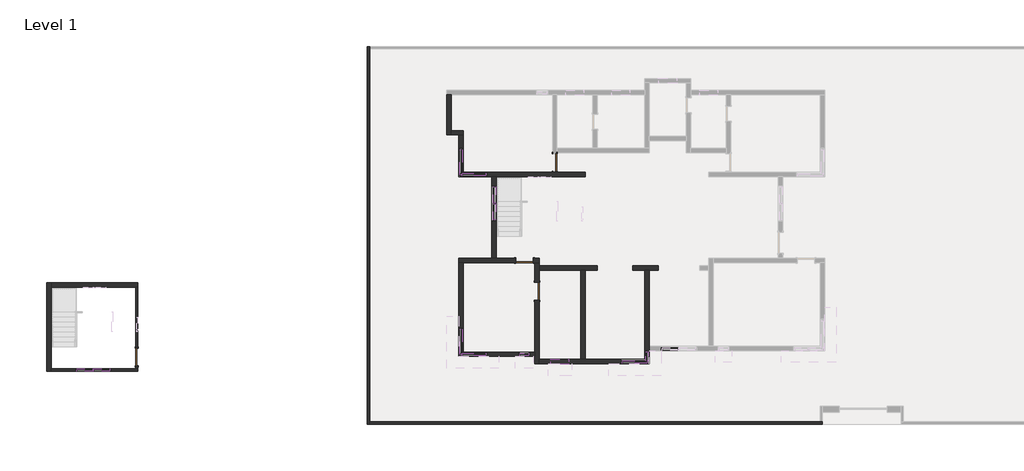
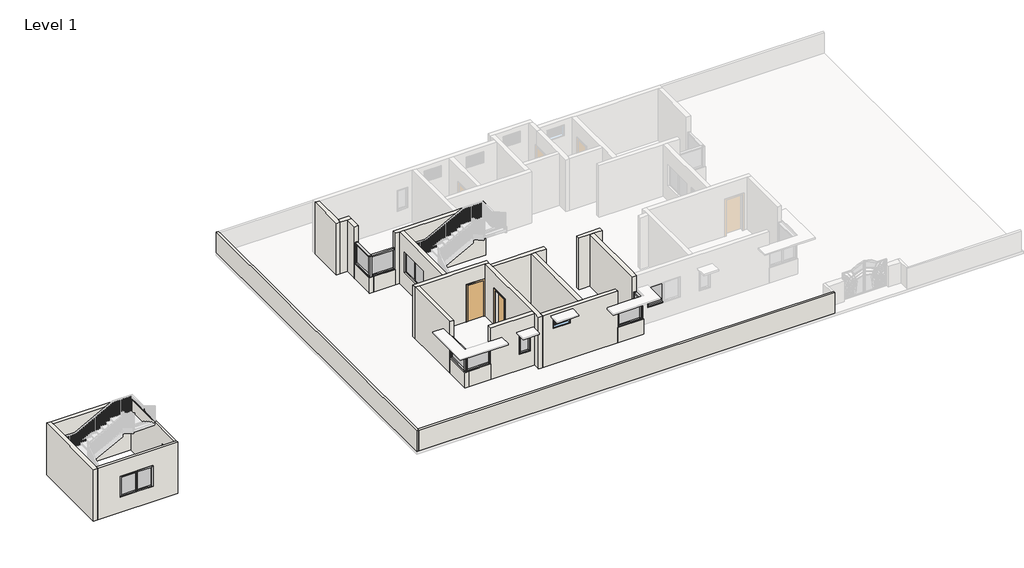
# One storey, part 1 of 9: 44 members, 26 walls, 12 plates, 4 doors, 1 window.
"""IFC4 building model written with IfcOpenShell, lengths in millimetres."""

from ifc_helpers import new_model, si_unit, frame, origin, origin_with_axes, place, context, project, spatial, polyline, outline, extrude, faceted_brep, transform, mapped, element, save
from components import single_flush_door_3_0ca8825f, single_flush_door_3_a90ba1ad, single_flush_door_3_305aa2a5, member_75074519, member_05917e3b, member_5783932f, member_d3e05364, member_2b49869a, member_9dc65bc2, member_c17f1be2, member_8d24a278, member_86d06fe4, system_panel_glazed_ffa60984, system_panel_glazed_87944ff9, system_panel_glazed_c8a97ecb, system_panel_glazed_fba3dfff, system_panel_glazed_90898af3, system_panel_glazed_d6173012, system_panel_glazed_7cebc396, system_panel_glazed_1bcf12e0, window_a18e4be4

model = new_model("IFC4")

# Units and contexts
model_context = context("Model", 3, world=origin())
ifc_project = project(units=[si_unit("LENGTHUNIT", "METRE", prefix="MILLI")], contexts=[model_context])

# Site, building, storey
site = spatial("IfcSite", under=ifc_project)
building = spatial("IfcBuilding", under=site)
storey = spatial("IfcBuildingStorey", under=building, Name="Level 1", Elevation=0.0)

# Doors
placement = place(None, origin())
single_flush_door_3_shape = single_flush_door_3_0ca8825f(model_context)
element("IfcDoor", 1, ObjectType="Single-Flush : door 3'", at=placement, inside=storey, context=model_context, shape_type="MappedRepresentation", body=[
    mapped(single_flush_door_3_shape, transform((-37991.8146233, 16182.7641869, 0.0), x_axis=(0.0, -1.0, 0.0), y_axis=(1.0, 0.0, 0.0), z_axis=(0.0, 0.0, 1.0))),
])
single_flush_door_3_2_shape = single_flush_door_3_a90ba1ad(model_context)
element("IfcDoor", 2, ObjectType="Single-Flush : door 3'", at=placement, inside=storey, context=model_context, shape_type="MappedRepresentation", body=[
    mapped(single_flush_door_3_2_shape, transform((-39541.2146233, 11158.0624892, 0.0), x_axis=(1.0, 0.0, 0.0), y_axis=(0.0, 1.0, 0.0), z_axis=(0.0, 0.0, 1.0))),
])
element("IfcDoor", 3, ObjectType="Single-Flush : door 3'", at=placement, inside=storey, context=model_context, shape_type="MappedRepresentation", body=[
    mapped(single_flush_door_3_2_shape, transform((-38906.2146233, 9583.2624892, 0.0), x_axis=(0.0, 1.0, 0.0), y_axis=(-1.0, 0.0, 0.0), z_axis=(0.0, 0.0, 1.0))),
])
single_flush_door_3_3_shape = single_flush_door_3_305aa2a5(model_context)
element("IfcDoor", 4, ObjectType="Single-Flush : door 3'", at=placement, inside=storey, context=model_context, shape_type="MappedRepresentation", body=[
    mapped(single_flush_door_3_3_shape, transform((-59414.6056789, 6214.5699577, 0.0), x_axis=(0.0, -1.0, 0.0), y_axis=(1.0, 0.0, 0.0), z_axis=(0.0, 0.0, 1.0))),
])

# Members
member_shape = member_75074519(model_context)
element("IfcMember", 5, ObjectType="Rectangular Mullion : 2.5\" x 5\" rectangular", at=placement, inside=storey, context=model_context, shape_type="MappedRepresentation", body=[
    mapped(member_shape, transform((-42808.6969478, 6281.2624892, 914.4), x_axis=(0.0, -1.0, 0.0), y_axis=(-1.0, 0.0, 0.0), z_axis=(0.0, 0.0, -1.0))),
])
element("IfcMember", 6, ObjectType="Rectangular Mullion : 2.5\" x 5\" rectangular", at=placement, inside=storey, context=model_context, shape_type="MappedRepresentation", body=[
    mapped(member_shape, transform((-41458.9146233, 6344.7624892, 914.4), x_axis=(1.0, 0.0, 0.0), y_axis=(0.0, -1.0, 0.0), z_axis=(0.0, 0.0, -1.0))),
])
element("IfcMember", 7, ObjectType="Rectangular Mullion : 2.5\" x 5\" rectangular", at=placement, inside=storey, context=model_context, shape_type="MappedRepresentation", body=[
    mapped(member_shape, transform((-42808.6027511, 15496.1692799, 914.4), x_axis=(0.0, -1.0, 0.0), y_axis=(-1.0, 0.0, 0.0), z_axis=(0.0, 0.0, -1.0))),
])
element("IfcMember", 8, ObjectType="Rectangular Mullion : 2.5\" x 5\" rectangular", at=placement, inside=storey, context=model_context, shape_type="MappedRepresentation", body=[
    mapped(member_shape, transform((-41458.9146233, 15559.6692799, 914.4), x_axis=(1.0, 0.0, 0.0), y_axis=(0.0, -1.0, 0.0), z_axis=(0.0, 0.0, -1.0))),
])
element("IfcMember", 9, ObjectType="Rectangular Mullion : 2.5\" x 5\" rectangular", at=placement, inside=storey, context=model_context, shape_type="MappedRepresentation", body=[
    mapped(member_shape, transform((-33191.2146233, 5950.984083, 914.4), x_axis=(1.0, 0.0, 0.0), y_axis=(0.0, -1.0, 0.0), z_axis=(0.0, 0.0, -1.0))),
])
element("IfcMember", 10, ObjectType="Rectangular Mullion : 2.5\" x 5\" rectangular", at=placement, inside=storey, context=model_context, shape_type="MappedRepresentation", body=[
    mapped(member_shape, transform((-33254.7146233, 6547.9624892, 914.4), x_axis=(0.0, 1.0, 0.0), y_axis=(1.0, 0.0, 0.0), z_axis=(0.0, 0.0, -1.0))),
])
element("IfcMember", 11, ObjectType="Rectangular Mullion : 2.5\" x 5\" rectangular", at=placement, inside=storey, context=model_context, shape_type="MappedRepresentation", body=[
    mapped(member_shape, transform((-41090.5055559, 15005.5684528, 914.4), x_axis=(0.0, 1.0, 0.0), y_axis=(1.0, 0.0, 0.0), z_axis=(0.0, 0.0, -1.0))),
])
element("IfcMember", 12, ObjectType="Rectangular Mullion : 2.5\" x 5\" rectangular", at=placement, inside=storey, context=model_context, shape_type="MappedRepresentation", body=[
    mapped(member_shape, transform((-60729.0556789, 5540.3224813, 914.4), x_axis=(1.0, 0.0, 0.0), y_axis=(0.0, -1.0, 0.0), z_axis=(0.0, 0.0, -1.0))),
])
element("IfcMember", 13, ObjectType="Rectangular Mullion : 2.5\" x 5\" rectangular", at=placement, inside=storey, context=model_context, shape_type="MappedRepresentation", body=[
    mapped(member_shape, transform((-39249.1146233, 6332.0624892, 914.4), x_axis=(1.0, 0.0, 0.0), y_axis=(0.0, -1.0, 0.0), z_axis=(0.0, 0.0, -1.0))),
])
element("IfcMember", 14, ObjectType="Rectangular Mullion : 2.5\" x 5\" rectangular", at=placement, inside=storey, context=model_context, shape_type="MappedRepresentation", body=[
    mapped(member_shape, transform((-42808.6969478, 7690.9624892, 2133.6), x_axis=(0.0, 1.0, 0.0), y_axis=(-1.0, 0.0, 0.0), z_axis=(0.0, 0.0, 1.0))),
])
element("IfcMember", 15, ObjectType="Rectangular Mullion : 2.5\" x 5\" rectangular", at=placement, inside=storey, context=model_context, shape_type="MappedRepresentation", body=[
    mapped(member_shape, transform((-42808.6969478, 6344.7624892, 2133.6), x_axis=(-1.0, 0.0, 0.0), y_axis=(0.0, -1.0, 0.0), z_axis=(0.0, 0.0, 1.0))),
])
element("IfcMember", 16, ObjectType="Rectangular Mullion : 2.5\" x 5\" rectangular", at=placement, inside=storey, context=model_context, shape_type="MappedRepresentation", body=[
    mapped(member_shape, transform((-42808.6027511, 16911.1624892, 2133.6), x_axis=(0.0, 1.0, 0.0), y_axis=(-1.0, 0.0, 0.0), z_axis=(0.0, 0.0, 1.0))),
])
element("IfcMember", 17, ObjectType="Rectangular Mullion : 2.5\" x 5\" rectangular", at=placement, inside=storey, context=model_context, shape_type="MappedRepresentation", body=[
    mapped(member_shape, transform((-42808.6027511, 15559.6692799, 2133.6), x_axis=(-1.0, 0.0, 0.0), y_axis=(0.0, -1.0, 0.0), z_axis=(0.0, 0.0, 1.0))),
])
element("IfcMember", 18, ObjectType="Rectangular Mullion : 2.5\" x 5\" rectangular", at=placement, inside=storey, context=model_context, shape_type="MappedRepresentation", body=[
    mapped(member_shape, transform((-34600.9146233, 5950.984083, 2133.6), x_axis=(-1.0, 0.0, 0.0), y_axis=(0.0, -1.0, 0.0), z_axis=(0.0, 0.0, 1.0))),
])
element("IfcMember", 19, ObjectType="Rectangular Mullion : 2.5\" x 5\" rectangular", at=placement, inside=storey, context=model_context, shape_type="MappedRepresentation", body=[
    mapped(member_shape, transform((-33254.7146233, 5950.984083, 2133.6), x_axis=(0.0, -1.0, 0.0), y_axis=(1.0, 0.0, 0.0), z_axis=(0.0, 0.0, 1.0))),
])
element("IfcMember", 20, ObjectType="Rectangular Mullion : 2.5\" x 5\" rectangular", at=placement, inside=storey, context=model_context, shape_type="MappedRepresentation", body=[
    mapped(member_shape, transform((-32543.5146233, 6636.8624892, 2133.6), x_axis=(-1.0, 0.0, 0.0), y_axis=(0.0, -1.0, 0.0), z_axis=(0.0, 0.0, 1.0))),
])
element("IfcMember", 21, ObjectType="Rectangular Mullion : 2.5\" x 5\" rectangular", at=placement, inside=storey, context=model_context, shape_type="MappedRepresentation", body=[
    mapped(member_shape, transform((-41090.5055559, 13177.3624892, 2133.6), x_axis=(0.0, -1.0, 0.0), y_axis=(1.0, 0.0, 0.0), z_axis=(0.0, 0.0, 1.0))),
])
element("IfcMember", 22, ObjectType="Rectangular Mullion : 2.5\" x 5\" rectangular", at=placement, inside=storey, context=model_context, shape_type="MappedRepresentation", body=[
    mapped(member_shape, transform((-62557.8556789, 5540.3224813, 2133.6), x_axis=(-1.0, 0.0, 0.0), y_axis=(0.0, -1.0, 0.0), z_axis=(0.0, 0.0, 1.0))),
])
element("IfcMember", 23, ObjectType="Rectangular Mullion : 2.5\" x 5\" rectangular", at=placement, inside=storey, context=model_context, shape_type="MappedRepresentation", body=[
    mapped(member_shape, transform((-39858.7146233, 6332.0624892, 2133.6), x_axis=(-1.0, 0.0, 0.0), y_axis=(0.0, -1.0, 0.0), z_axis=(0.0, 0.0, 1.0))),
])
member_2_shape = member_05917e3b(model_context)
element("IfcMember", 24, ObjectType="Rectangular Mullion : 2.5\" x 5\" rectangular", at=placement, inside=storey, context=model_context, shape_type="MappedRepresentation", body=[
    mapped(member_2_shape, transform((-41522.4146233, 6344.7624892, 2133.6), x_axis=(0.0, 0.0, 1.0), y_axis=(0.0, -1.0, 0.0), z_axis=(1.0, 0.0, 0.0))),
])
element("IfcMember", 25, ObjectType="Rectangular Mullion : 2.5\" x 5\" rectangular", at=placement, inside=storey, context=model_context, shape_type="MappedRepresentation", body=[
    mapped(member_2_shape, transform((-41522.4146233, 15559.6692799, 2133.6), x_axis=(0.0, 0.0, 1.0), y_axis=(0.0, -1.0, 0.0), z_axis=(1.0, 0.0, 0.0))),
])
element("IfcMember", 26, ObjectType="Rectangular Mullion : 2.5\" x 5\" rectangular", at=placement, inside=storey, context=model_context, shape_type="MappedRepresentation", body=[
    mapped(member_2_shape, transform((-42745.1969478, 6344.7624892, 914.4), x_axis=(0.0, 0.0, -1.0), y_axis=(0.0, -1.0, 0.0), z_axis=(-1.0, 0.0, 0.0))),
])
element("IfcMember", 27, ObjectType="Rectangular Mullion : 2.5\" x 5\" rectangular", at=placement, inside=storey, context=model_context, shape_type="MappedRepresentation", body=[
    mapped(member_2_shape, transform((-42745.1027511, 15559.6692799, 914.4), x_axis=(0.0, 0.0, -1.0), y_axis=(0.0, -1.0, 0.0), z_axis=(-1.0, 0.0, 0.0))),
])
member_3_shape = member_5783932f(model_context)
element("IfcMember", 28, ObjectType="Rectangular Mullion : 2.5\" x 5\" rectangular", at=placement, inside=storey, context=model_context, shape_type="MappedRepresentation", body=[
    mapped(member_3_shape, transform((-42808.6969478, 6344.7624892, 2133.6), x_axis=(0.0, 0.0, 1.0), y_axis=(-1.0, 0.0, 0.0), z_axis=(0.0, -1.0, 0.0))),
])
element("IfcMember", 29, ObjectType="Rectangular Mullion : 2.5\" x 5\" rectangular", at=placement, inside=storey, context=model_context, shape_type="MappedRepresentation", body=[
    mapped(member_3_shape, transform((-33254.7146233, 5950.984083, 2133.6), x_axis=(0.0, 0.0, 1.0), y_axis=(0.0, -1.0, 0.0), z_axis=(1.0, 0.0, 0.0))),
])
element("IfcMember", 30, ObjectType="Rectangular Mullion : 2.5\" x 5\" rectangular", at=placement, inside=storey, context=model_context, shape_type="MappedRepresentation", body=[
    mapped(member_3_shape, transform((-42808.6969478, 7627.4624892, 914.4), x_axis=(0.0, 0.0, -1.0), y_axis=(-1.0, 0.0, 0.0), z_axis=(0.0, 1.0, 0.0))),
])
element("IfcMember", 31, ObjectType="Rectangular Mullion : 2.5\" x 5\" rectangular", at=placement, inside=storey, context=model_context, shape_type="MappedRepresentation", body=[
    mapped(member_3_shape, transform((-34537.4146233, 5950.984083, 914.4), x_axis=(0.0, 0.0, -1.0), y_axis=(0.0, -1.0, 0.0), z_axis=(-1.0, 0.0, 0.0))),
])
member_4_shape = member_d3e05364(model_context)
element("IfcMember", 32, ObjectType="Rectangular Mullion : 2.5\" x 5\" rectangular", at=placement, inside=storey, context=model_context, shape_type="MappedRepresentation", body=[
    mapped(member_4_shape, transform((-42808.6027511, 15559.6692799, 2133.6), x_axis=(0.0, 0.0, 1.0), y_axis=(-1.0, 0.0, 0.0), z_axis=(0.0, -1.0, 0.0))),
])
element("IfcMember", 33, ObjectType="Rectangular Mullion : 2.5\" x 5\" rectangular", at=placement, inside=storey, context=model_context, shape_type="MappedRepresentation", body=[
    mapped(member_4_shape, transform((-42808.6027511, 16847.6624892, 914.4), x_axis=(0.0, 0.0, -1.0), y_axis=(-1.0, 0.0, 0.0), z_axis=(0.0, 1.0, 0.0))),
])
member_5_shape = member_2b49869a(model_context)
element("IfcMember", 34, ObjectType="Rectangular Mullion : 2.5\" x 5\" rectangular", at=placement, inside=storey, context=model_context, shape_type="MappedRepresentation", body=[
    mapped(member_5_shape, transform((-41090.5055559, 14091.465471, 914.4), x_axis=(0.0, 1.0, 0.0), y_axis=(1.0, 0.0, 0.0), z_axis=(0.0, 0.0, -1.0))),
])
element("IfcMember", 35, ObjectType="Rectangular Mullion : 2.5\" x 5\" rectangular", at=placement, inside=storey, context=model_context, shape_type="MappedRepresentation", body=[
    mapped(member_5_shape, transform((-61643.4556789, 5540.3224813, 914.4), x_axis=(1.0, 0.0, 0.0), y_axis=(0.0, -1.0, 0.0), z_axis=(0.0, 0.0, -1.0))),
])
member_6_shape = member_9dc65bc2(model_context)
element("IfcMember", 36, ObjectType="Rectangular Mullion : 2.5\" x 5\" rectangular", at=placement, inside=storey, context=model_context, shape_type="MappedRepresentation", body=[
    mapped(member_6_shape, transform((-33254.7146233, 6484.4624892, 2133.6), x_axis=(0.0, 0.0, 1.0), y_axis=(1.0, 0.0, 0.0), z_axis=(0.0, 1.0, 0.0))),
])
element("IfcMember", 37, ObjectType="Rectangular Mullion : 2.5\" x 5\" rectangular", at=placement, inside=storey, context=model_context, shape_type="MappedRepresentation", body=[
    mapped(member_6_shape, transform((-33254.7146233, 6014.484083, 914.4), x_axis=(0.0, 0.0, -1.0), y_axis=(1.0, 0.0, 0.0), z_axis=(0.0, -1.0, 0.0))),
])
member_7_shape = member_c17f1be2(model_context)
element("IfcMember", 38, ObjectType="Rectangular Mullion : 2.5\" x 5\" rectangular", at=placement, inside=storey, context=model_context, shape_type="MappedRepresentation", body=[
    mapped(member_7_shape, transform((-60792.5556789, 5540.3224813, 2133.6), x_axis=(0.0, 0.0, 1.0), y_axis=(0.0, -1.0, 0.0), z_axis=(1.0, 0.0, 0.0))),
])
element("IfcMember", 39, ObjectType="Rectangular Mullion : 2.5\" x 5\" rectangular", at=placement, inside=storey, context=model_context, shape_type="MappedRepresentation", body=[
    mapped(member_7_shape, transform((-61675.2056789, 5540.3224813, 2133.6), x_axis=(0.0, 0.0, 1.0), y_axis=(0.0, -1.0, 0.0), z_axis=(1.0, 0.0, 0.0))),
])
element("IfcMember", 40, ObjectType="Rectangular Mullion : 2.5\" x 5\" rectangular", at=placement, inside=storey, context=model_context, shape_type="MappedRepresentation", body=[
    mapped(member_7_shape, transform((-32480.0146233, 6636.8624892, 914.4), x_axis=(0.0, 0.0, -1.0), y_axis=(0.0, -1.0, 0.0), z_axis=(-1.0, 0.0, 0.0))),
])
element("IfcMember", 41, ObjectType="Rectangular Mullion : 2.5\" x 5\" rectangular", at=placement, inside=storey, context=model_context, shape_type="MappedRepresentation", body=[
    mapped(member_7_shape, transform((-62494.3556789, 5540.3224813, 914.4), x_axis=(0.0, 0.0, -1.0), y_axis=(0.0, -1.0, 0.0), z_axis=(-1.0, 0.0, 0.0))),
])
element("IfcMember", 42, ObjectType="Rectangular Mullion : 2.5\" x 5\" rectangular", at=placement, inside=storey, context=model_context, shape_type="MappedRepresentation", body=[
    mapped(member_7_shape, transform((-61611.7056789, 5540.3224813, 914.4), x_axis=(0.0, 0.0, -1.0), y_axis=(0.0, -1.0, 0.0), z_axis=(-1.0, 0.0, 0.0))),
])
member_8_shape = member_8d24a278(model_context)
element("IfcMember", 43, ObjectType="Rectangular Mullion : 2.5\" x 5\" rectangular", at=placement, inside=storey, context=model_context, shape_type="MappedRepresentation", body=[
    mapped(member_8_shape, transform((-41090.5055559, 14942.0684528, 2133.6), x_axis=(0.0, 0.0, 1.0), y_axis=(1.0, 0.0, 0.0), z_axis=(0.0, 1.0, 0.0))),
])
element("IfcMember", 44, ObjectType="Rectangular Mullion : 2.5\" x 5\" rectangular", at=placement, inside=storey, context=model_context, shape_type="MappedRepresentation", body=[
    mapped(member_8_shape, transform((-41090.5055559, 14059.715471, 2133.6), x_axis=(0.0, 0.0, 1.0), y_axis=(1.0, 0.0, 0.0), z_axis=(0.0, 1.0, 0.0))),
])
element("IfcMember", 45, ObjectType="Rectangular Mullion : 2.5\" x 5\" rectangular", at=placement, inside=storey, context=model_context, shape_type="MappedRepresentation", body=[
    mapped(member_8_shape, transform((-41090.5055559, 13240.8624892, 914.4), x_axis=(0.0, 0.0, -1.0), y_axis=(1.0, 0.0, 0.0), z_axis=(0.0, -1.0, 0.0))),
])
element("IfcMember", 46, ObjectType="Rectangular Mullion : 2.5\" x 5\" rectangular", at=placement, inside=storey, context=model_context, shape_type="MappedRepresentation", body=[
    mapped(member_8_shape, transform((-41090.5055559, 14123.215471, 914.4), x_axis=(0.0, 0.0, -1.0), y_axis=(1.0, 0.0, 0.0), z_axis=(0.0, -1.0, 0.0))),
])
member_9_shape = member_86d06fe4(model_context)
element("IfcMember", 47, ObjectType="Rectangular Mullion : 2.5\" x 5\" rectangular", at=placement, inside=storey, context=model_context, shape_type="MappedRepresentation", body=[
    mapped(member_9_shape, transform((-39312.6146233, 6332.0624892, 2133.6), x_axis=(0.0, 0.0, 1.0), y_axis=(0.0, -1.0, 0.0), z_axis=(1.0, 0.0, 0.0))),
])
element("IfcMember", 48, ObjectType="Rectangular Mullion : 2.5\" x 5\" rectangular", at=placement, inside=storey, context=model_context, shape_type="MappedRepresentation", body=[
    mapped(member_9_shape, transform((-39795.2146233, 6332.0624892, 914.4), x_axis=(0.0, 0.0, -1.0), y_axis=(0.0, -1.0, 0.0), z_axis=(-1.0, 0.0, 0.0))),
])

# Plates
system_panel_glazed_shape = system_panel_glazed_ffa60984(model_context)
element("IfcPlate", 49, ObjectType="System Panel : Glazed", at=placement, inside=storey, context=model_context, shape_type="MappedRepresentation", body=[
    mapped(system_panel_glazed_shape, transform((-42133.8057856, 6344.7624892, 977.9), x_axis=(1.0, 0.0, 0.0), y_axis=(0.0, 1.0, 0.0), z_axis=(0.0, 0.0, 1.0))),
])
system_panel_glazed_2_shape = system_panel_glazed_87944ff9(model_context)
element("IfcPlate", 50, ObjectType="System Panel : Glazed", at=placement, inside=storey, context=model_context, shape_type="MappedRepresentation", body=[
    mapped(system_panel_glazed_2_shape, transform((-42808.6969478, 6986.1124892, 977.9), x_axis=(0.0, -1.0, 0.0), y_axis=(1.0, 0.0, 0.0), z_axis=(0.0, 0.0, 1.0))),
])
element("IfcPlate", 51, ObjectType="System Panel : Glazed", at=placement, inside=storey, context=model_context, shape_type="MappedRepresentation", body=[
    mapped(system_panel_glazed_2_shape, transform((-33896.0646233, 5950.984083, 977.9), x_axis=(1.0, 0.0, 0.0), y_axis=(0.0, 1.0, 0.0), z_axis=(0.0, 0.0, 1.0))),
])
system_panel_glazed_3_shape = system_panel_glazed_c8a97ecb(model_context)
element("IfcPlate", 52, ObjectType="System Panel : Glazed", at=placement, inside=storey, context=model_context, shape_type="MappedRepresentation", body=[
    mapped(system_panel_glazed_3_shape, transform((-42133.7586872, 15559.6692799, 977.9), x_axis=(1.0, 0.0, 0.0), y_axis=(0.0, 1.0, 0.0), z_axis=(0.0, 0.0, 1.0))),
])
system_panel_glazed_4_shape = system_panel_glazed_fba3dfff(model_context)
element("IfcPlate", 53, ObjectType="System Panel : Glazed", at=placement, inside=storey, context=model_context, shape_type="MappedRepresentation", body=[
    mapped(system_panel_glazed_4_shape, transform((-42808.6027511, 16203.6658846, 977.9), x_axis=(0.0, -1.0, 0.0), y_axis=(1.0, 0.0, 0.0), z_axis=(0.0, 0.0, 1.0))),
])
system_panel_glazed_5_shape = system_panel_glazed_90898af3(model_context)
element("IfcPlate", 54, ObjectType="System Panel : Glazed", at=placement, inside=storey, context=model_context, shape_type="MappedRepresentation", body=[
    mapped(system_panel_glazed_5_shape, transform((-33254.7146233, 6249.4732861, 977.9), x_axis=(0.0, 1.0, 0.0), y_axis=(-1.0, 0.0, 0.0), z_axis=(0.0, 0.0, 1.0))),
])
system_panel_glazed_6_shape = system_panel_glazed_d6173012(model_context)
element("IfcPlate", 55, ObjectType="System Panel : Glazed", at=placement, inside=storey, context=model_context, shape_type="MappedRepresentation", body=[
    mapped(system_panel_glazed_6_shape, transform((-32070.4396233, 6636.8624892, 977.9), x_axis=(1.0, 0.0, 0.0), y_axis=(0.0, 1.0, 0.0), z_axis=(0.0, 0.0, 1.0))),
])
element("IfcPlate", 56, ObjectType="System Panel : Glazed", at=placement, inside=storey, context=model_context, shape_type="MappedRepresentation", body=[
    mapped(system_panel_glazed_6_shape, transform((-62084.7806789, 5540.3224813, 977.9), x_axis=(1.0, 0.0, 0.0), y_axis=(0.0, 1.0, 0.0), z_axis=(0.0, 0.0, 1.0))),
])
element("IfcPlate", 57, ObjectType="System Panel : Glazed", at=placement, inside=storey, context=model_context, shape_type="MappedRepresentation", body=[
    mapped(system_panel_glazed_6_shape, transform((-61202.1306789, 5540.3224813, 977.9), x_axis=(1.0, 0.0, 0.0), y_axis=(0.0, 1.0, 0.0), z_axis=(0.0, 0.0, 1.0))),
])
system_panel_glazed_7_shape = system_panel_glazed_7cebc396(model_context)
element("IfcPlate", 58, ObjectType="System Panel : Glazed", at=placement, inside=storey, context=model_context, shape_type="MappedRepresentation", body=[
    mapped(system_panel_glazed_7_shape, transform((-41090.5055559, 13650.2889801, 977.9), x_axis=(0.0, 1.0, 0.0), y_axis=(-1.0, 0.0, 0.0), z_axis=(0.0, 0.0, 1.0))),
])
element("IfcPlate", 59, ObjectType="System Panel : Glazed", at=placement, inside=storey, context=model_context, shape_type="MappedRepresentation", body=[
    mapped(system_panel_glazed_7_shape, transform((-41090.5055559, 14532.6419619, 977.9), x_axis=(0.0, 1.0, 0.0), y_axis=(-1.0, 0.0, 0.0), z_axis=(0.0, 0.0, 1.0))),
])
system_panel_glazed_8_shape = system_panel_glazed_1bcf12e0(model_context)
element("IfcPlate", 60, ObjectType="System Panel : Glazed", at=placement, inside=storey, context=model_context, shape_type="MappedRepresentation", body=[
    mapped(system_panel_glazed_8_shape, transform((-39553.9146233, 6332.0624892, 977.9), x_axis=(1.0, 0.0, 0.0), y_axis=(0.0, 1.0, 0.0), z_axis=(0.0, 0.0, 1.0))),
])

# Walls
element("IfcWall", 61, at=placement, inside=storey, context=model_context, shape_type="Brep", body=[
    faceted_brep([(-47478.7146233, 2776.0624892, 0.0), (-47478.7146233, 2890.3624892, 0.0), (-47478.7146233, 22016.5624892, 0.0), (-47478.7146233, 22130.8624892, 0.0), (-47478.7146233, 22130.8624892, 1219.2), (-47478.7146233, 22016.5624892, 1219.2), (-47478.7146233, 2890.3624892, 1219.2), (-47478.7146233, 2776.0624892, 1219.2), (-47593.0146233, 2776.0624892, 0.0), (-47593.0146233, 2776.0624892, 1219.2), (-47593.0146233, 22130.8624892, 1219.2), (-47593.0146233, 22130.8624892, 0.0)], [[[0, 1, 2, 3, 4, 5, 6, 7]], [[8, 9, 10, 11]], [[3, 2, 1, 0, 8, 11]], [[7, 6, 5, 4, 10, 9]], [[4, 3, 11, 10]], [[0, 7, 9, 8]]]),
])
element("IfcWall", 62, at=placement, inside=storey, context=model_context, shape_type="Brep", body=[
    faceted_brep([(-47478.7146233, 2776.0624892, 0.0), (-24275.8146233, 2776.0624892, 0.0), (-24275.8146233, 2776.0624892, 1219.2), (-47478.7146233, 2776.0624892, 1219.2), (-47478.7146233, 2890.3624892, 0.0), (-47478.7146233, 2890.3624892, 1219.2), (-24390.1146233, 2890.3624892, 1219.2), (-24275.8146233, 2890.3624892, 1219.2), (-24275.8146233, 2890.3624892, 0.0), (-24390.1146233, 2890.3624892, 0.0)], [[[0, 1, 2, 3]], [[4, 5, 6, 7, 8, 9]], [[1, 0, 4, 9, 8]], [[3, 2, 7, 6, 5]], [[0, 3, 5, 4]], [[2, 1, 8, 7]]]),
])
element("IfcWall", 63, ObjectType="Generic - 5\"", at=placement, inside=storey, context=model_context, shape_type="Brep", body=[
    faceted_brep([(-63814.6636189, 5497.0199577, 0.0), (-59357.4556789, 5497.0199577, 0.0), (-59357.4556789, 5497.0199577, 3048.0), (-63814.6636189, 5497.0199577, 3048.0), (-62557.8556789, 5497.0199577, 914.4), (-62557.8556789, 5497.0199577, 2133.6), (-60729.0556789, 5497.0199577, 2133.6), (-60729.0556789, 5497.0199577, 914.4), (-59357.4556789, 5611.3199577, 0.0), (-59471.7556789, 5611.3199577, 0.0), (-63814.6636189, 5611.3199577, 0.0), (-63814.6636189, 5611.3199577, 3048.0), (-59471.7556789, 5611.3199577, 3048.0), (-59357.4556789, 5611.3199577, 3048.0), (-62557.8556789, 5611.3199577, 2133.6), (-62557.8556789, 5611.3199577, 914.4), (-60729.0556789, 5611.3199577, 914.4), (-60729.0556789, 5611.3199577, 2133.6)], [[[0, 1, 2, 3], [4, 5, 6, 7]], [[8, 9, 10, 11, 12, 13], [14, 15, 16, 17]], [[1, 0, 10, 9, 8]], [[2, 1, 8, 13]], [[0, 3, 11, 10]], [[4, 15, 14, 5]], [[5, 14, 17, 6]], [[6, 17, 16, 7]], [[15, 4, 7, 16]], [[3, 2, 13, 12, 11]]]),
])
element("IfcWall", 64, ObjectType="Generic - 5\"", at=placement, inside=storey, context=model_context, shape_type="Brep", body=[
    faceted_brep([(-59357.4556789, 5611.3199577, 0.0), (-59357.4556789, 5757.3699577, 0.0), (-59357.4556789, 5757.3699577, 2133.6), (-59357.4556789, 6671.7699577, 2133.6), (-59357.4556789, 6671.7699577, 0.0), (-59357.4556789, 9802.3199577, 0.0), (-59357.4556789, 9802.3199577, 3048.0), (-59357.4556789, 5611.3199577, 3048.0), (-59471.7556789, 5757.3699577, 2133.6), (-59471.7556789, 5757.3699577, 0.0), (-59471.7556789, 5611.3199577, 0.0), (-59471.7556789, 5611.3199577, 3048.0), (-59471.7556789, 9802.3199577, 3048.0), (-59471.7556789, 9802.3199577, 0.0), (-59471.7556789, 6671.7699577, 0.0), (-59471.7556789, 6671.7699577, 2133.6), (-59471.2636189, 5611.3199577, 3048.0), (-59471.2636189, 9802.3199577, 3048.0), (-59471.2636189, 7516.3199577, 3048.0)], [[[0, 1, 2, 3, 4, 5, 6, 7]], [[8, 9, 10, 11, 12, 13, 14, 15]], [[14, 13, 5, 4]], [[10, 9, 1, 0]], [[0, 7, 16, 11, 10]], [[6, 5, 13, 12, 17]], [[2, 1, 9, 8]], [[3, 2, 8, 15]], [[4, 3, 15, 14]], [[7, 6, 17, 18, 16]], [[17, 12, 11, 16, 18]]]),
])
element("IfcWall", 65, ObjectType="WALL 9\" 2", at=placement, inside=storey, context=model_context, shape_type="Brep", body=[
    faceted_brep([(-43516.3146233, 19654.3624892, 0.0), (-43516.3146233, 17596.9624892, 0.0), (-43516.3146233, 17596.9624892, 3048.0), (-43516.3146233, 19654.3624892, 3048.0), (-43287.7146233, 19654.3624892, 0.0), (-43287.7146233, 19654.3624892, 3048.0), (-43287.7146233, 17825.5624892, 3048.0), (-43287.7146233, 17596.9624892, 3048.0), (-43287.7146233, 17596.9624892, 0.0), (-43287.7146233, 17825.5624892, 0.0)], [[[0, 1, 2, 3]], [[4, 5, 6, 7, 8, 9]], [[1, 0, 4, 9, 8]], [[3, 2, 7, 6, 5]], [[0, 3, 5, 4]], [[2, 1, 8, 7]]]),
])
element("IfcWall", 66, ObjectType="WALL 9\" 2", at=placement, inside=storey, context=model_context, shape_type="Brep", body=[
    faceted_brep([(-43287.7146233, 17596.9624892, 0.0), (-42906.7146233, 17596.9624892, 0.0), (-42678.1146233, 17596.9624892, 0.0), (-42678.1146233, 17596.9624892, 3048.0), (-42906.7146233, 17596.9624892, 3048.0), (-43287.7146233, 17596.9624892, 3048.0), (-43287.7146233, 17825.5624892, 0.0), (-43287.7146233, 17825.5624892, 3048.0), (-42678.1146233, 17825.5624892, 3048.0), (-42678.1146233, 17825.5624892, 0.0)], [[[0, 1, 2, 3, 4, 5]], [[6, 7, 8, 9]], [[2, 1, 0, 6, 9]], [[5, 4, 3, 8, 7]], [[0, 5, 7, 6]], [[3, 2, 9, 8]]]),
])
element("IfcWall", 67, ObjectType="WALL 9\" 2", at=placement, inside=storey, context=model_context, shape_type="Brep", body=[
    faceted_brep([(-42906.7146233, 17596.9624892, 0.0), (-42906.7146233, 16911.1624892, 0.0), (-42906.7146233, 16911.1624892, 914.4), (-42906.7146233, 16911.1624892, 2133.6), (-42906.7146233, 16911.1624892, 3048.0), (-42906.7146233, 17596.9624892, 3048.0), (-42678.1146233, 17596.9624892, 0.0), (-42678.1146233, 17596.9624892, 3048.0), (-42678.1146233, 16911.1624892, 3048.0), (-42678.1146233, 16911.1624892, 2133.6), (-42678.1146233, 16911.1624892, 914.4), (-42678.1146233, 16911.1624892, 0.0)], [[[0, 1, 2, 3, 4, 5]], [[6, 7, 8, 9, 10, 11]], [[1, 0, 6, 11]], [[5, 4, 8, 7]], [[0, 5, 7, 6]], [[1, 11, 10, 9, 8, 4, 3, 2]]]),
])
element("IfcWall", 68, ObjectType="WALL 9\" 2", at=placement, inside=storey, context=model_context, shape_type="Brep", body=[
    faceted_brep([(-41458.9146233, 15454.3658846, 3048.0), (-41458.9146233, 15454.3658846, 2133.6), (-41458.9146233, 15454.3658846, 914.4), (-41458.9146233, 15454.3658846, 0.0), (-41230.3146233, 15454.3658846, 0.0), (-41001.7146233, 15454.3658846, 0.0), (-36429.7146233, 15454.3658846, 0.0), (-36429.7146233, 15454.3658846, 3048.0), (-41001.7146233, 15454.3658846, 3048.0), (-41230.3146233, 15454.3658846, 3048.0), (-41458.9146233, 15682.9658846, 0.0), (-41458.9146233, 15682.9658846, 914.4), (-41458.9146233, 15682.9658846, 2133.6), (-41458.9146233, 15682.9658846, 3048.0), (-38106.1146233, 15682.9658846, 3048.0), (-37877.5146233, 15682.9658846, 3048.0), (-36429.7146233, 15682.9658846, 3048.0), (-36429.7146233, 15682.9658846, 0.0), (-37877.5146233, 15682.9658846, 0.0), (-38106.1146233, 15682.9658846, 0.0)], [[[0, 1, 2, 3, 4, 5, 6, 7, 8, 9]], [[10, 11, 12, 13, 14, 15, 16, 17, 18, 19]], [[6, 5, 4, 3, 10, 19, 18, 17]], [[7, 6, 17, 16]], [[0, 9, 8, 7, 16, 15, 14, 13]], [[0, 13, 12, 11, 10, 3, 2, 1]]]),
])
element("IfcWall", 69, ObjectType="WALL 9\" 2", at=placement, inside=storey, context=model_context, shape_type="SweptSolid", body=[
    extrude(outline(polyline([(15454.3658846, 0.0), (11272.3624892, 0.0), (11272.3624892, 3048.0), (15454.3658846, 3048.0), (15454.3658846, 0.0)]), holes=[polyline([(13177.3624892, 2133.6), (13177.3624892, 914.4), (15005.5684528, 914.4), (15005.5684528, 2133.6), (13177.3624892, 2133.6)])]), frame((-41230.3146233, 0.0, 0.0), z_axis=(1.0, 0.0, 0.0), x_axis=(0.0, 1.0, 0.0)), (0.0, 0.0, 1.0), 228.6),
])
element("IfcWall", 70, ObjectType="WALL 9\" 2", at=placement, inside=storey, context=model_context, shape_type="Brep", body=[
    faceted_brep([(-39084.0146233, 11043.7624892, 2133.6), (-39084.0146233, 11043.7624892, 0.0), (-39020.5146233, 11043.7624892, 0.0), (-38791.9146233, 11043.7624892, 0.0), (-38791.9146233, 11043.7624892, 3048.0), (-39020.5146233, 11043.7624892, 3048.0), (-42678.1146233, 11043.7624892, 3048.0), (-42906.7146233, 11043.7624892, 3048.0), (-42906.7146233, 11043.7624892, 0.0), (-42678.1146233, 11043.7624892, 0.0), (-39998.4146233, 11043.7624892, 0.0), (-39998.4146233, 11043.7624892, 2133.6), (-38791.9146233, 11272.3624892, 0.0), (-39084.0146233, 11272.3624892, 0.0), (-39084.0146233, 11272.3624892, 2133.6), (-39998.4146233, 11272.3624892, 2133.6), (-39998.4146233, 11272.3624892, 0.0), (-41001.7146233, 11272.3624892, 0.0), (-41230.3146233, 11272.3624892, 0.0), (-42906.7146233, 11272.3624892, 0.0), (-42906.7146233, 11272.3624892, 3048.0), (-41230.3146233, 11272.3624892, 3048.0), (-41001.7146233, 11272.3624892, 3048.0), (-38791.9146233, 11272.3624892, 3048.0)], [[[0, 1, 2, 3, 4, 5, 6, 7, 8, 9, 10, 11]], [[12, 13, 14, 15, 16, 17, 18, 19, 20, 21, 22, 23]], [[10, 9, 8, 19, 18, 17, 16]], [[3, 2, 1, 13, 12]], [[7, 6, 5, 4, 23, 22, 21, 20]], [[4, 3, 12, 23]], [[8, 7, 20, 19]], [[14, 13, 1, 0]], [[15, 14, 0, 11]], [[16, 15, 11, 10]]]),
])
element("IfcWall", 71, ObjectType="WALL 9\" 2", at=placement, inside=storey, context=model_context, shape_type="Brep", body=[
    faceted_brep([(-39020.5146233, 11043.7624892, 0.0), (-39020.5146233, 10040.4624892, 0.0), (-39020.5146233, 10040.4624892, 2133.6), (-39020.5146233, 9126.0624892, 2133.6), (-39020.5146233, 9126.0624892, 0.0), (-39020.5146233, 6471.7624892, 0.0), (-39020.5146233, 6243.1624892, 0.0), (-39020.5146233, 5862.084083, 0.0), (-39020.5146233, 5862.084083, 3048.0), (-39020.5146233, 6243.1624892, 3048.0), (-39020.5146233, 6471.7624892, 3048.0), (-39020.5146233, 11043.7624892, 3048.0), (-38791.9146233, 10040.4624892, 2133.6), (-38791.9146233, 10040.4624892, 0.0), (-38791.9146233, 10662.7624892, 0.0), (-38791.9146233, 10891.3624892, 0.0), (-38791.9146233, 11043.7624892, 0.0), (-38791.9146233, 11043.7624892, 3048.0), (-38791.9146233, 10891.3624892, 3048.0), (-38791.9146233, 10662.7624892, 3048.0), (-38791.9146233, 6090.684083, 3048.0), (-38791.9146233, 5862.084083, 3048.0), (-38791.9146233, 5862.084083, 0.0), (-38791.9146233, 6090.684083, 0.0), (-38791.9146233, 9126.0624892, 0.0), (-38791.9146233, 9126.0624892, 2133.6)], [[[0, 1, 2, 3, 4, 5, 6, 7, 8, 9, 10, 11]], [[12, 13, 14, 15, 16, 17, 18, 19, 20, 21, 22, 23, 24, 25]], [[16, 15, 14, 13, 1, 0]], [[24, 23, 22, 7, 6, 5, 4]], [[11, 10, 9, 8, 21, 20, 19, 18, 17]], [[0, 11, 17, 16]], [[8, 7, 22, 21]], [[2, 1, 13, 12]], [[3, 2, 12, 25]], [[4, 3, 25, 24]]]),
])
element("IfcWall", 72, ObjectType="WALL 9\" 2", at=placement, inside=storey, context=model_context, shape_type="Brep", body=[
    faceted_brep([(-42906.7146233, 11043.7624892, 0.0), (-42906.7146233, 7690.9624892, 0.0), (-42906.7146233, 7690.9624892, 914.4), (-42906.7146233, 7690.9624892, 2133.6), (-42906.7146233, 7690.9624892, 3048.0), (-42906.7146233, 11043.7624892, 3048.0), (-42678.1146233, 11043.7624892, 0.0), (-42678.1146233, 11043.7624892, 3048.0), (-42678.1146233, 7690.9624892, 3048.0), (-42678.1146233, 7690.9624892, 2133.6), (-42678.1146233, 7690.9624892, 914.4), (-42678.1146233, 7690.9624892, 0.0)], [[[0, 1, 2, 3, 4, 5]], [[6, 7, 8, 9, 10, 11]], [[1, 0, 6, 11]], [[5, 4, 8, 7]], [[0, 5, 7, 6]], [[1, 11, 10, 9, 8, 4, 3, 2]]]),
])
element("IfcWall", 73, ObjectType="WALL 9\" 2", at=placement, inside=storey, context=model_context, shape_type="Brep", body=[
    faceted_brep([(-41458.9146233, 6243.1624892, 0.0), (-39020.5146233, 6243.1624892, 0.0), (-39020.5146233, 6243.1624892, 3048.0), (-41458.9146233, 6243.1624892, 3048.0), (-41458.9146233, 6243.1624892, 2133.6), (-41458.9146233, 6243.1624892, 914.4), (-39858.7146233, 6243.1624892, 914.4), (-39858.7146233, 6243.1624892, 2133.6), (-39249.1146233, 6243.1624892, 2133.6), (-39249.1146233, 6243.1624892, 914.4), (-39020.5146233, 6471.7624892, 0.0), (-41458.9146233, 6471.7624892, 0.0), (-41458.9146233, 6471.7624892, 914.4), (-41458.9146233, 6471.7624892, 2133.6), (-41458.9146233, 6471.7624892, 3048.0), (-39020.5146233, 6471.7624892, 3048.0), (-39858.7146233, 6471.7624892, 2133.6), (-39858.7146233, 6471.7624892, 914.4), (-39249.1146233, 6471.7624892, 914.4), (-39249.1146233, 6471.7624892, 2133.6)], [[[0, 1, 2, 3, 4, 5], [6, 7, 8, 9]], [[10, 11, 12, 13, 14, 15], [16, 17, 18, 19]], [[1, 0, 11, 10]], [[3, 2, 15, 14]], [[2, 1, 10, 15]], [[3, 14, 13, 12, 11, 0, 5, 4]], [[6, 17, 16, 7]], [[7, 16, 19, 8]], [[8, 19, 18, 9]], [[17, 6, 9, 18]]]),
])
element("IfcWall", 74, ObjectType="WALL 9\" 2", at=placement, inside=storey, context=model_context, shape_type="Brep", body=[
    faceted_brep([(-38791.9146233, 5862.084083, 0.0), (-34600.9146233, 5862.084083, 0.0), (-34600.9146233, 5862.084083, 914.4), (-34600.9146233, 5862.084083, 2133.6), (-34600.9146233, 5862.084083, 3048.0), (-38791.9146233, 5862.084083, 3048.0), (-38195.0146233, 5862.084083, 2743.2), (-37280.6146233, 5862.084083, 2743.2), (-37280.6146233, 5862.084083, 2133.6), (-38195.0146233, 5862.084083, 2133.6), (-38791.9146233, 6090.684083, 0.0), (-38791.9146233, 6090.684083, 3048.0), (-36658.3146233, 6090.684083, 3048.0), (-36429.7146233, 6090.684083, 3048.0), (-34600.9146233, 6090.684083, 3048.0), (-34600.9146233, 6090.684083, 2133.6), (-34600.9146233, 6090.684083, 914.4), (-34600.9146233, 6090.684083, 0.0), (-36429.7146233, 6090.684083, 0.0), (-36658.3146233, 6090.684083, 0.0), (-38195.0146233, 6090.684083, 2743.2), (-38195.0146233, 6090.684083, 2133.6), (-37280.6146233, 6090.684083, 2133.6), (-37280.6146233, 6090.684083, 2743.2)], [[[0, 1, 2, 3, 4, 5], [6, 7, 8, 9]], [[10, 11, 12, 13, 14, 15, 16, 17, 18, 19], [20, 21, 22, 23]], [[1, 0, 10, 19, 18, 17]], [[5, 4, 14, 13, 12, 11]], [[0, 5, 11, 10]], [[1, 17, 16, 15, 14, 4, 3, 2]], [[21, 20, 6, 9]], [[22, 21, 9, 8]], [[23, 22, 8, 7]], [[20, 23, 7, 6]]]),
])
element("IfcWall", 75, ObjectType="WALL 9\" 2", at=placement, inside=storey, context=model_context, shape_type="SweptSolid", body=[
    extrude(outline(polyline([(-36429.7146233, 10662.7624892), (-36429.7146233, 6090.684083), (-36658.3146233, 6090.684083), (-36658.3146233, 10662.7624892), (-36429.7146233, 10662.7624892)])), origin_with_axes(), (0.0, 0.0, 1.0), 3048.0),
])
element("IfcWall", 76, ObjectType="WALL 9\" 2", at=placement, inside=storey, context=model_context, shape_type="Brep", body=[
    faceted_brep([(-38791.9146233, 10662.7624892, 0.0), (-36658.3146233, 10662.7624892, 0.0), (-36429.7146233, 10662.7624892, 0.0), (-35820.1146233, 10662.7624892, 0.0), (-35820.1146233, 10662.7624892, 3048.0), (-36429.7146233, 10662.7624892, 3048.0), (-36658.3146233, 10662.7624892, 3048.0), (-38791.9146233, 10662.7624892, 3048.0), (-38791.9146233, 10891.3624892, 0.0), (-38791.9146233, 10891.3624892, 3048.0), (-35820.1146233, 10891.3624892, 3048.0), (-35820.1146233, 10891.3624892, 0.0)], [[[0, 1, 2, 3, 4, 5, 6, 7]], [[8, 9, 10, 11]], [[3, 2, 1, 0, 8, 11]], [[4, 3, 11, 10]], [[7, 6, 5, 4, 10, 9]], [[0, 7, 9, 8]]]),
])
element("IfcWall", 77, ObjectType="WALL 9\" 2", at=placement, inside=storey, context=model_context, shape_type="Brep", body=[
    faceted_brep([(-33152.7428374, 6547.9624892, 3048.0), (-33152.7428374, 6547.9624892, 0.0), (-33152.7428374, 6776.5624892, 0.0), (-33152.7428374, 10662.7624892, 0.0), (-33152.7428374, 10662.7624892, 3048.0), (-33152.7428374, 6776.5624892, 3048.0), (-33381.3428374, 6547.9624892, 0.0), (-33381.3428374, 6547.9624892, 3048.0), (-33381.3428374, 10662.7624892, 3048.0), (-33381.3428374, 10662.7624892, 0.0), (-33153.1146233, 6547.9624892, 0.0), (-33153.1146233, 6547.9624892, 3048.0)], [[[0, 1, 2, 3, 4, 5]], [[6, 7, 8, 9]], [[3, 2, 1, 10, 6, 9]], [[0, 5, 4, 8, 7, 11]], [[4, 3, 9, 8]], [[0, 11, 7, 6, 10, 1]]]),
])
element("IfcWall", 78, ObjectType="WALL 9\" 2", at=placement, inside=storey, context=model_context, shape_type="Brep", body=[
    faceted_brep([(-64043.2636189, 10030.9199577, 0.0), (-64043.2636189, 5497.0199577, 0.0), (-64043.2636189, 5497.0199577, 3048.0), (-64043.2636189, 10030.9199577, 3048.0), (-63814.6636189, 10030.9199577, 0.0), (-63814.6636189, 10030.9199577, 3048.0), (-63814.6636189, 9802.3199577, 3048.0), (-63814.6636189, 6754.3199577, 3048.0), (-63814.6636189, 5611.3199577, 3048.0), (-63814.6636189, 5497.0199577, 3048.0), (-63814.6636189, 5497.0199577, 0.0), (-63814.6636189, 5611.3199577, 0.0), (-63814.6636189, 9802.3199577, 0.0)], [[[0, 1, 2, 3]], [[4, 5, 6, 7, 8, 9, 10, 11, 12]], [[1, 0, 4, 12, 11, 10]], [[0, 3, 5, 4]], [[2, 1, 10, 9]], [[3, 2, 9, 8, 7, 6, 5]]]),
])
element("IfcWall", 79, ObjectType="WALL 9\" 2", at=placement, inside=storey, context=model_context, shape_type="Brep", body=[
    faceted_brep([(-63814.6636189, 9802.3199577, 0.0), (-59471.7556789, 9802.3199577, 0.0), (-59357.4556789, 9802.3199577, 0.0), (-59357.4556789, 9802.3199577, 3048.0), (-59471.2636189, 9802.3199577, 3048.0), (-59471.7556789, 9802.3199577, 3048.0), (-63814.6636189, 9802.3199577, 3048.0), (-63814.6636189, 10030.9199577, 0.0), (-63814.6636189, 10030.9199577, 3048.0), (-59357.4556789, 10030.9199577, 3048.0), (-59357.4556789, 10030.9199577, 0.0)], [[[0, 1, 2, 3, 4, 5, 6]], [[7, 8, 9, 10]], [[2, 1, 0, 7, 10]], [[0, 6, 8, 7]], [[3, 2, 10, 9]], [[6, 5, 4, 3, 9, 8]]]),
])
element("IfcWall", 80, ObjectType="WALL 9\" 2", at=placement, inside=storey, context=model_context, shape_type="Brep", body=[
    faceted_brep([(-33991.3146233, 10662.7624892, 0.0), (-33381.3428374, 10662.7624892, 0.0), (-33152.7428374, 10662.7624892, 0.0), (-32695.9146233, 10662.7624892, 0.0), (-32695.9146233, 10662.7624892, 3048.0), (-33152.7428374, 10662.7624892, 3048.0), (-33381.3428374, 10662.7624892, 3048.0), (-33991.3146233, 10662.7624892, 3048.0), (-33991.3146233, 10891.3624892, 0.0), (-33991.3146233, 10891.3624892, 3048.0), (-32695.9146233, 10891.3624892, 3048.0), (-32695.9146233, 10891.3624892, 0.0)], [[[0, 1, 2, 3, 4, 5, 6, 7]], [[8, 9, 10, 11]], [[3, 2, 1, 0, 8, 11]], [[4, 3, 11, 10]], [[7, 6, 5, 4, 10, 9]], [[0, 7, 9, 8]]]),
])
element("IfcWall", 81, ObjectType="wall 3'", at=placement, inside=storey, context=model_context, shape_type="Brep", body=[
    faceted_brep([(-42906.7146233, 7690.9624892, 0.0), (-42906.7146233, 6243.1624892, 0.0), (-42906.7146233, 6243.1624892, 914.4), (-42906.7146233, 7690.9624892, 914.4), (-42678.1146233, 7690.9624892, 0.0), (-42678.1146233, 7690.9624892, 914.4), (-42678.1146233, 6471.7624892, 914.4), (-42678.1146233, 6243.1624892, 914.4), (-42678.1146233, 6243.1624892, 0.0), (-42678.1146233, 6471.7624892, 0.0)], [[[0, 1, 2, 3]], [[4, 5, 6, 7, 8, 9]], [[1, 0, 4, 9, 8]], [[3, 2, 7, 6, 5]], [[0, 3, 5, 4]], [[2, 1, 8, 7]]]),
])
element("IfcWall", 82, ObjectType="wall 3'", at=placement, inside=storey, context=model_context, shape_type="SweptSolid", body=[
    extrude(outline(polyline([(-41458.9146233, 6243.1624892), (-42678.1146233, 6243.1624892), (-42678.1146233, 6471.7624892), (-41458.9146233, 6471.7624892), (-41458.9146233, 6243.1624892)])), origin_with_axes(), (0.0, 0.0, 1.0), 914.4),
])
element("IfcWall", 83, ObjectType="wall 3'", at=placement, inside=storey, context=model_context, shape_type="Brep", body=[
    faceted_brep([(-42906.7146233, 16911.1624892, 0.0), (-42906.7146233, 15454.3658846, 0.0), (-42906.7146233, 15454.3658846, 914.4), (-42906.7146233, 16911.1624892, 914.4), (-42678.1146233, 16911.1624892, 0.0), (-42678.1146233, 16911.1624892, 914.4), (-42678.1146233, 15682.9658846, 914.4), (-42678.1146233, 15454.3658846, 914.4), (-42678.1146233, 15454.3658846, 0.0), (-42678.1146233, 15682.9658846, 0.0)], [[[0, 1, 2, 3]], [[4, 5, 6, 7, 8, 9]], [[1, 0, 4, 9, 8]], [[3, 2, 7, 6, 5]], [[0, 3, 5, 4]], [[2, 1, 8, 7]]]),
])
element("IfcWall", 84, ObjectType="wall 3'", at=placement, inside=storey, context=model_context, shape_type="SweptSolid", body=[
    extrude(outline(polyline([(-41458.9146233, 15454.3658846), (-42678.1146233, 15454.3658846), (-42678.1146233, 15682.9658846), (-41458.9146233, 15682.9658846), (-41458.9146233, 15454.3658846)])), origin_with_axes(), (0.0, 0.0, 1.0), 914.4),
])
element("IfcWall", 85, ObjectType="wall 3'", at=placement, inside=storey, context=model_context, shape_type="Brep", body=[
    faceted_brep([(-34600.9146233, 5862.084083, 0.0), (-33153.1146233, 5862.084083, 0.0), (-33153.1146233, 5862.084083, 914.4), (-34600.9146233, 5862.084083, 914.4), (-34600.9146233, 6090.684083, 0.0), (-34600.9146233, 6090.684083, 914.4), (-33381.7146233, 6090.684083, 914.4), (-33153.1146233, 6090.684083, 914.4), (-33153.1146233, 6090.684083, 0.0), (-33381.7146233, 6090.684083, 0.0)], [[[0, 1, 2, 3]], [[4, 5, 6, 7, 8, 9]], [[1, 0, 4, 9, 8]], [[3, 2, 7, 6, 5]], [[0, 3, 5, 4]], [[2, 1, 8, 7]]]),
])
element("IfcWall", 86, ObjectType="wall 3'", at=placement, inside=storey, context=model_context, shape_type="Brep", body=[
    faceted_brep([(-33153.1146233, 6090.684083, 0.0), (-33153.1146233, 6547.9624892, 0.0), (-33153.1146233, 6547.9624892, 914.4), (-33153.1146233, 6090.684083, 914.4), (-33381.7146233, 6090.684083, 0.0), (-33381.7146233, 6090.684083, 914.4), (-33381.7146233, 6547.9624892, 914.4), (-33381.7146233, 6547.9624892, 0.0), (-33381.3428374, 6547.9624892, 0.0)], [[[0, 1, 2, 3]], [[4, 5, 6, 7]], [[1, 0, 4, 7, 8]], [[3, 2, 6, 5]], [[0, 3, 5, 4]], [[2, 1, 8, 7, 6]]]),
])

# Window
window_shape = window_a18e4be4(model_context)
element("IfcWindow", 87, ObjectType="Window-Louvers : 36\" x 24\"", at=placement, inside=storey, context=model_context, shape_type="MappedRepresentation", body=[
    mapped(window_shape, transform((-37737.8146233, 5982.734083, 1219.2), x_axis=(1.0, 0.0, 0.0), y_axis=(0.0, 1.0, 0.0), z_axis=(0.0, 0.0, 1.0))),
])

save(model, "model.ifc")

# Revit data of these elements
# Type "Single-Flush : door 3'"
#   Type Mark = "8"
#   Construction Type Id = "MDOOR"
#   Assembly Code = "C1020"
#   Analytic Construction = "Metal"
#   Thickness = 0' - 2"
#   Heat Transfer Coefficient (U) = 0.651978 BTU/(h·ft²·°F)
#   Height = 7' - 0"
#   Trim Projection Ext = 0' - 1"
#   Trim Projection Int = 0' - 1"
#   Trim Width = 0' - 3"
#   Width = 3' - 0"
#   Define Thermal Properties by = 1
#   Door Material = Door - Panel
#   Frame Material = Door - Frame
#   Visual Light Transmittance = 0
#   Solar Heat Gain Coefficient = 0
#   Function = (empty or 0)
#   Wall Closure = (empty or 0)
# Type "Rectangular Mullion : 2.5\" x 5\" rectangular"
#   built-in parameter 1007304 = 0.416667 (stored number, unit not read)
#   built-in parameter 1007301 = 0.104167 (stored number, unit not read)
#   built-in parameter 1007300 = 0.104167 (stored number, unit not read)
# Type "System Panel : Glazed"
#   Construction Type Id = "GSP4R"
#   Analytic Construction = "1/8 in Pilkington single glazing"
#   Visual Light Transmittance = 0.9
#   Solar Heat Gain Coefficient = 0.86
#   Heat Transfer Coefficient (U) = 1.18115 BTU/(h·ft²·°F)
#   Define Thermal Properties by = 1
# Type
#   Assembly Code = "B2010"
#   Layers, outside or top first: 0' - 4 1/2" no material (function 1)
# Type "Generic - 5\""
#   Assembly Code = "B2010"
#   Layers, outside or top first: 0' - 4 1/2" no material (function 1)
# Type "WALL 9\" 2"
#   Assembly Code = "B2010"
#   Layers, outside or top first: 0' - 9" no material (function 1)
# Type "wall 3'"
#   Assembly Code = "B2010"
#   Layers, outside or top first: 0' - 9" no material (function 1)
# Type "Window-Louvers : 36\" x 24\""
#   Type Mark = "18"
#   Construction Type Id = "GSP4R"
#   Assembly Code = "B20"
#   Analytic Construction = "1/8 in Pilkington single glazing"
#   Visual Light Transmittance = 0.9
#   Thermal Resistance (R) = 1.53941 (h·ft²·°F)/BTU
#   Solar Heat Gain Coefficient = 0.78
#   Max Height = 1' - 11.74264"
#   Height = 2' - 0"
#   Heat Transfer Coefficient (U) = 0.6496 BTU/(h·ft²·°F)
#   Blade Width [instance default] = 2' - 10 1/2"
#   Blade Vertical Thickness = 0' - 0.35355"
#   Blade Thickness = 0' - 0 1/4"
#   Blade Spacing = 0' - 1 1/2"
#   Blade Height = 0' - 1.85355"
#   Blade Depth = 0' - 3"
#   Blade Angle = 45.00°
#   Default Sill Height = 3' - 0"
#   Trim Projection_Exterior = 0' - 0 1/2"
#   Trim Projection_Interior = 0' - 0 1/2"
#   Trim Width_Exterior = 0' - 1 1/2"
#   Trim Width_Interior = 0' - 1 1/2"
#   Width = 3' - 0"
#   Max Blade Count = 12
#   Define Thermal Properties by = 1
#   Blade Count = 12
#   Frame Material = Birch
#   Louver Material = Birch
#   Trim Exterior Material = Birch
#   Trim Interior Material = Birch
#   Wall Closure = (empty or 0)
# Elements 1, 2, 3, 4 (IfcDoor, "Single-Flush : door 3'")
#   Phase Created = New Construction
#   Materials on its faces: "Door - Frame", "Door - Panel"
# Elements 5, 6, 7, 8, 9, 10, 11, 12, 13, 14, 15, 16, 17, 18, 19, 20, 21, 22, 23, 24, 25, 26, 27, 28, 29, 30, 31, 32, 33, 34, 35, 36, 37, 38, 39, 40, 41, 42, 43, 44, 45, 46, 47, 48 (IfcMember, "Rectangular Mullion : 2.5\" x 5\" rectangular")
#   Phase Created = New Construction
#   Materials on its faces: "Aluminum"
# Elements 49, 50, 51, 52, 53, 54, 55, 56, 57, 58, 59, 60 (IfcPlate, "System Panel : Glazed")
#   Phase Created = New Construction
#   Materials on its faces: "Glass"
# Elements 61, 62 (IfcWall)
#   Top Offset = 0' - 0"
#   Base Offset = 0' - 0"
#   Unconnected Height = 4' - 0"
#   wall height = 4' - 0"
#   Phase Created = New Construction
#   Base Constraint = Level 1
#   Materials on its faces: "Clad - White", "Default Wall"
# Elements 63, 64 (IfcWall, "Generic - 5\"")
#   Top Offset = 0' - 0"
#   Base Offset = 0' - 0"
#   Unconnected Height = 10' - 0"
#   wall height = 10' - 0"
#   Phase Created = New Construction
#   Base Constraint = Level 1
#   Materials on its faces: "Default Wall"
# Elements 65, 66, 67, 68, 69, 70, 71, 72, 73, 74, 77 (IfcWall, "WALL 9\" 2")
#   Top Offset = 0' - 0"
#   Base Offset = 0' - 0"
#   Unconnected Height = 10' - 0"
#   wall height = 10' - 0"
#   Phase Created = New Construction
#   Base Constraint = Level 1
#   Materials on its faces: "Default Wall", "Wood Planks"
# Elements 75, 76, 78, 79, 80 (IfcWall, "WALL 9\" 2")
#   Top Offset = 0' - 0"
#   Base Offset = 0' - 0"
#   Unconnected Height = 10' - 0"
#   wall height = 10' - 0"
#   Phase Created = New Construction
#   Base Constraint = Level 1
#   Materials on its faces: "Default Wall"
# Elements 81, 82, 83, 84, 85, 86 (IfcWall, "wall 3'")
#   Top Offset = 0' - 0"
#   Base Offset = 0' - 0"
#   Unconnected Height = 3' - 0"
#   wall height = 3' - 0"
#   Phase Created = New Construction
#   Base Constraint = Level 1
#   Materials on its faces: "Default Wall", "Wood Planks"
# Element 87 (IfcWindow, "Window-Louvers : 36\" x 24\"")
#   Mark = "5"
#   Blade Width = 2' - 10 1/2"
#   Phase Created = New Construction
#   Materials on its faces: "Birch"
# Materials
#   "Door - Panel": class "Wood", colour RGB 210 159 95, transparency 0, Cost = 0
#   "Door - Frame": colour RGB 118 70 51, transparency 0, Cost = 0
#   "Birch": class "Wood", colour RGB 224 178 126, transparency 0, Description = "Betula Alleghaniensis", Cost = 0
#   "Aluminum": class "Metal", colour RGB 247 247 247, transparency 0, Description = "Aluminum 6061", Cost = 0
#   "Glass": class "Glass", colour RGB 0 128 192, transparency 0.75, Description = "Soda Lime Glass", Cost = 0
#   "Clad - White": class "Wood", colour RGB 242 242 238, transparency 0, Cost = 0
#   "Default Wall": colour RGB 128 128 128, transparency 0, Cost = 0
#   "Wood Planks": class "Wood", colour RGB 193 160 115, transparency 0, Description = "Physical material.", Cost = 0
